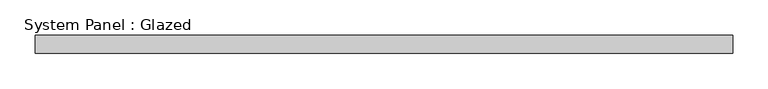
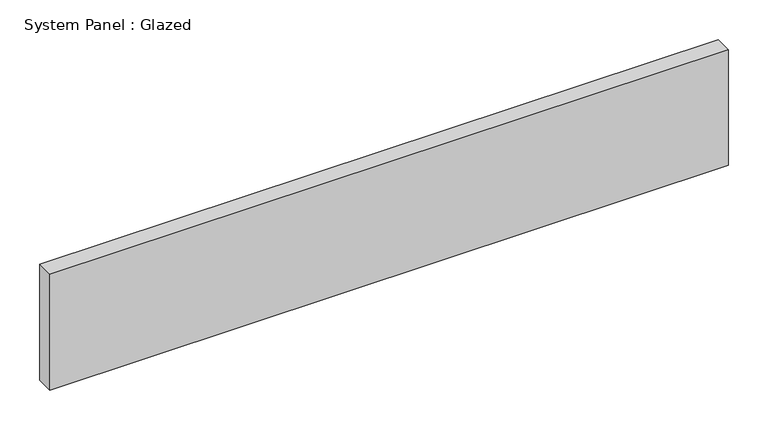
"""IFC4 building model written with IfcOpenShell, lengths in millimetres: plate geometry, System Panel : Glazed."""

from ifc_helpers import new_model, si_unit, origin, origin_with_axes, place, context, project, spatial, polyline, outline, extrude, source, transform, mapped, element, save


def system_panel_glazed_471f9198(model_context):
    return source(origin(), model_context, "Body", "SweptSolid", [
        extrude(outline(polyline([(493.1833332, 19.05), (-493.1833332, 19.05), (-493.1833332, 44.45), (493.1833332, 44.45), (493.1833332, 19.05)])), origin_with_axes(), (0.0, 0.0, 1.0), 177.8),
    ])


if __name__ == "__main__":
    model = new_model("IFC4")
    model_context = context("Model", 3, world=origin())
    ifc_project = project(units=[si_unit("LENGTHUNIT", "METRE", prefix="MILLI")], contexts=[model_context])
    site = spatial("IfcSite", under=ifc_project)
    building = spatial("IfcBuilding", under=site)
    placement = place(None, origin())
    system_panel_glazed_shape = system_panel_glazed_471f9198(model_context)
    element("IfcPlate", 1, ObjectType="System Panel : Glazed", at=placement, inside=building, context=model_context, shape_type="MappedRepresentation", body=[
        mapped(system_panel_glazed_shape, transform((0.0, 0.0, 0.0), x_axis=(1.0, 0.0, 0.0), y_axis=(0.0, 1.0, 0.0), z_axis=(0.0, 0.0, 1.0))),
    ])
    save(model, "model.ifc")

# Revit data of these elements
# Type "System Panel : Glazed"
#   Construction Type Id = "GSP4R"
#   Analytic Construction = "1/8 in Pilkington single glazing"
#   Visual Light Transmittance = 0.9
#   Solar Heat Gain Coefficient = 0.86
#   Heat Transfer Coefficient (U) = 1.18115 BTU/(h·ft²·°F)
#   Define Thermal Properties by = 1
# Element 1 (IfcPlate, "System Panel : Glazed")
#   Materials on its faces: "Glass"
# Materials
#   "Glass": class "Glass", colour RGB 0 128 192, transparency 0.75, Description = "Soda Lime Glass", Cost = 0
